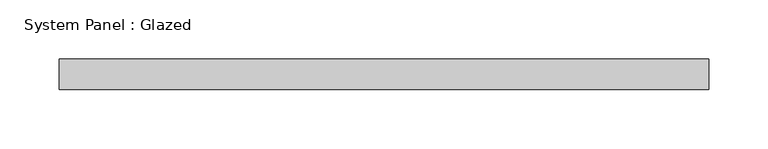
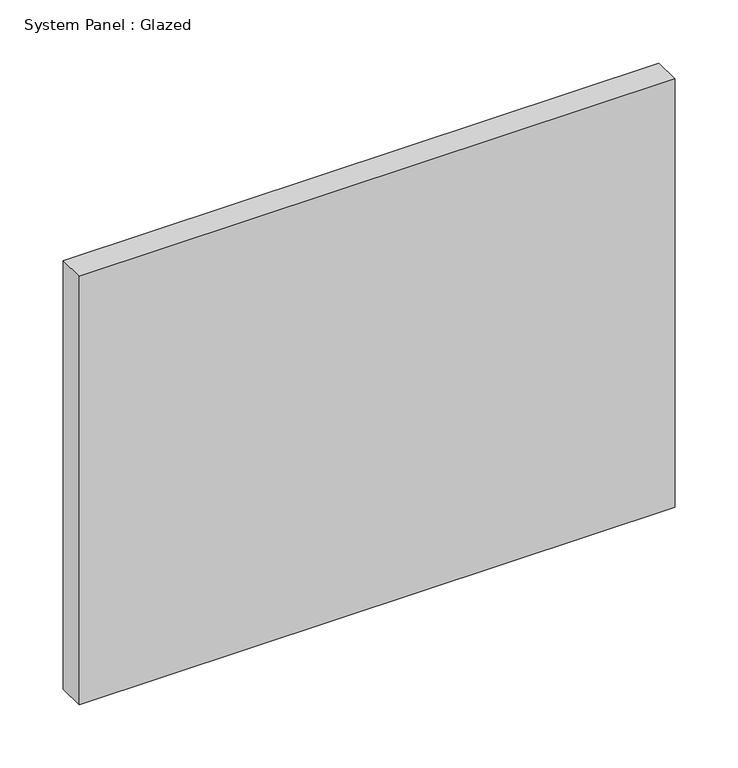
"""IFC4 building model written with IfcOpenShell, lengths in millimetres: plate geometry, System Panel : Glazed."""

from ifc_helpers import new_model, si_unit, origin, origin_with_axes, place, context, project, spatial, polyline, outline, extrude, source, transform, mapped, element, save


def system_panel_glazed_09ca6336(model_context):
    return source(origin(), model_context, "Body", "SweptSolid", [
        extrude(outline(polyline([(273.05, 19.05), (-273.05, 19.05), (-273.05, 44.45), (273.05, 44.45), (273.05, 19.05)])), origin_with_axes(), (0.0, 0.0, 1.0), 414.8666667),
    ])


if __name__ == "__main__":
    model = new_model("IFC4")
    model_context = context("Model", 3, world=origin())
    ifc_project = project(units=[si_unit("LENGTHUNIT", "METRE", prefix="MILLI")], contexts=[model_context])
    site = spatial("IfcSite", under=ifc_project)
    building = spatial("IfcBuilding", under=site)
    placement = place(None, origin())
    system_panel_glazed_shape = system_panel_glazed_09ca6336(model_context)
    element("IfcPlate", 1, ObjectType="System Panel : Glazed", at=placement, inside=building, context=model_context, shape_type="MappedRepresentation", body=[
        mapped(system_panel_glazed_shape, transform((0.0, 0.0, 0.0), x_axis=(1.0, 0.0, 0.0), y_axis=(0.0, 1.0, 0.0), z_axis=(0.0, 0.0, 1.0))),
    ])
    save(model, "model.ifc")

# Revit data of these elements
# Type "System Panel : Glazed"
#   Construction Type Id = "GSP4R"
#   Analytic Construction = "1/8 in Pilkington single glazing"
#   Visual Light Transmittance = 0.9
#   Solar Heat Gain Coefficient = 0.86
#   Heat Transfer Coefficient (U) = 1.18115 BTU/(h·ft²·°F)
#   Define Thermal Properties by = 1
# Element 1 (IfcPlate, "System Panel : Glazed")
#   Materials on its faces: "Glass"
# Materials
#   "Glass": class "Glass", colour RGB 0 128 192, transparency 0.75, Description = "Soda Lime Glass", Cost = 0
